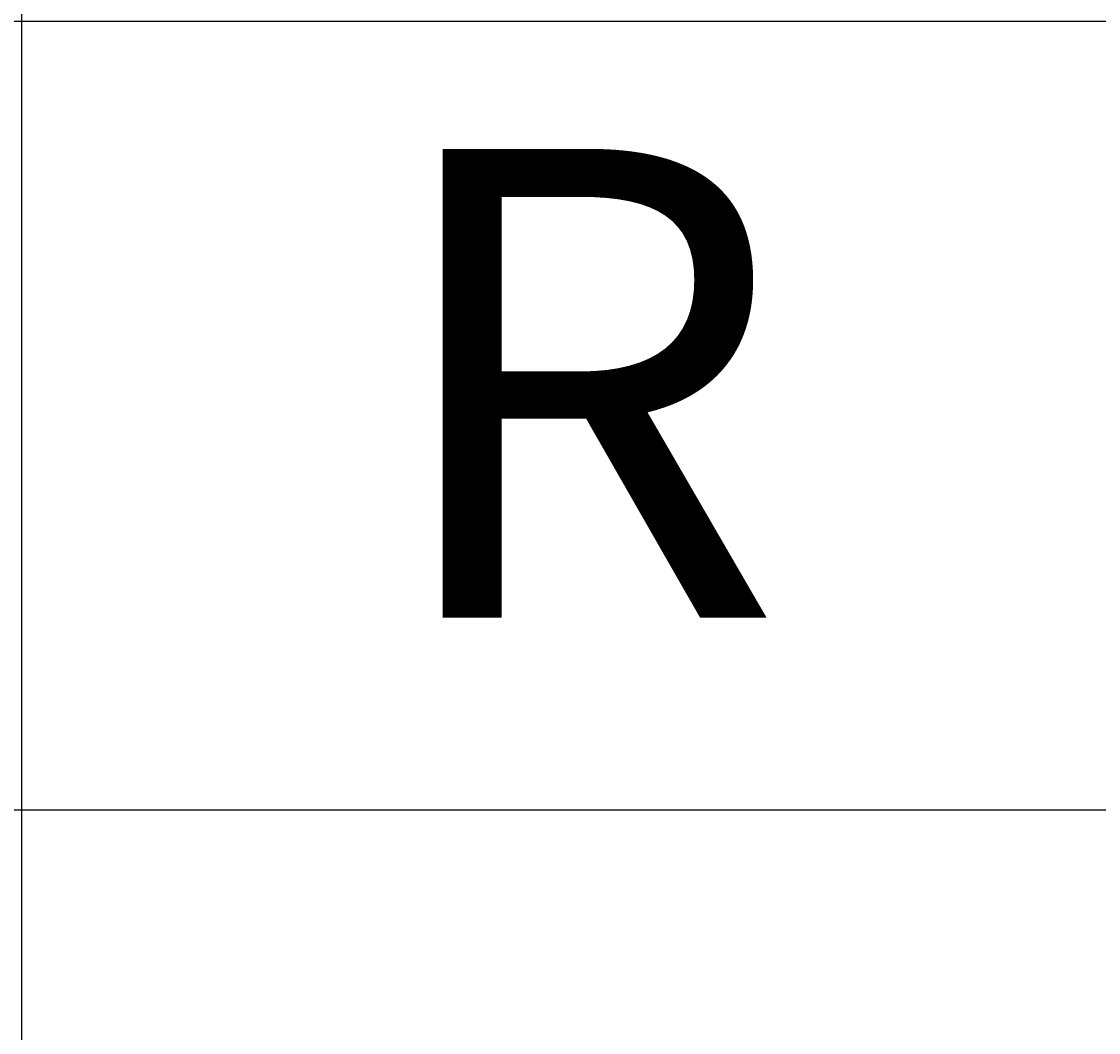
# Model space of a CAD drawing. Units: inches. Extents: x 35362 to 73946, y 43607 to 67532.
# Tile 134 of 134: x 67327 to 67834, y 59646 to 60122. Entities that reach past the tile are written whole.
import ezdxf

# ---------------------------------------------------------------- set-up
doc = ezdxf.new("R2010")
doc.units = ezdxf.units.IN
doc.header["$MEASUREMENT"] = 0
for name, color, linetype, lineweight in [('A-ANNO-DIMS', 2, 'Continuous', 18), ('E-ANNO-TEXT', 5, 'Continuous', 18), ('E-WIRE', 3, 'Continuous', 25)]:
    doc.layers.add(name, color=color, linetype=linetype, lineweight=lineweight)
doc.styles.get("Standard").update_dxf_attribs({"font": 'arial.ttf'})
doc.dimstyles.get("Standard").update_dxf_attribs({"dimtxt": 0.18, "dimasz": 0.18, "dimexe": 0.18, "dimexo": 0.0625, "dimgap": 0.09, "dimtad": 0, "dimtih": 1, "dimtoh": 1, "dimdec": 4, "dimzin": 0, "dimdsep": 46, "dimtxsty": 'Standard', "dimcen": 0.09, "dimadec": 0, "dimazin": 0, "dimtfac": 1, "dimtdec": 4, "dimtofl": 0, "dimtmove": 0, "dimatfit": 3, "dimfxl": 1, "dimtolj": 1, "dimtzin": 0, "dimarcsym": 0})

# ---------------------------------------------------------------- blocks, each defined once
blk = doc.blocks.new('*D8')
at = {"layer": 'A-ANNO-DIMS', "color": 0, "lineweight": -2, "transparency": 16777216}
for p, q in [((66271.28651900003, 65771.51172800003), (73945.82566600003, 65771.51172800003)), ((73945.64566600005, 65771.33172800003), (73945.64566600005, 59737.03093663782)), ((73945.64566600005, 53702.36633900002), (73945.64566600005, 59736.66713036224)), ((72185.70816600003, 53702.18633900003), (73945.82566600003, 53702.18633900003))]:
    blk.add_line(p, q, dxfattribs=at)
at = {"layer": 'A-ANNO-DIMS', "color": 0, "transparency": 16777216}
for points in [[(73945.61566600006, 65771.33172800003), (73945.67566600005, 65771.33172800003), (73945.64566600005, 65771.51172800003)], [(73945.61566600006, 53702.36633900002), (73945.67566600005, 53702.36633900002), (73945.64566600005, 53702.18633900003)]]:
    blk.add_solid(points, dxfattribs=at)
at = {"layer": 'Defpoints', "color": 0, "transparency": 16777216}
for p in [(66271.22401900003, 65771.51172800003), (73945.64566600005, 65771.51172800003), (72185.64566600003, 53702.18633900003)]:
    blk.add_point(p, dxfattribs=at)
at = {"layer": 'A-ANNO-DIMS', "color": 0, "transparency": 16777216, "insert": (73945.64566600005, 59736.84903349999), "char_height": 0.18, "attachment_point": 5}
blk.add_mtext('\\A1;12069', dxfattribs=at)
blk = doc.blocks.new('*D35')
at = {"layer": 'A-ANNO-DIMS', "color": 0, "lineweight": -2, "transparency": 16777216}
for p, q in [((61240.907336, 59185.206457), (61240.907336, 67531.691728)), ((61241.08733599999, 67531.51172799998), (64780.42646373397, 67531.51172799998)), ((68320.69076200001, 67531.51172799998), (64781.35163426603, 67531.51172799998)), ((68320.870762, 60122.408832), (68320.870762, 67531.691728))]:
    blk.add_line(p, q, dxfattribs=at)
at = {"layer": 'A-ANNO-DIMS', "color": 0, "transparency": 16777216}
for points in [[(61241.08733599999, 67531.541728), (61241.08733599999, 67531.481728), (61240.907336, 67531.51172799998)], [(68320.69076200001, 67531.541728), (68320.69076200001, 67531.481728), (68320.870762, 67531.51172799998)]]:
    blk.add_solid(points, dxfattribs=at)
at = {"layer": 'Defpoints', "color": 0, "transparency": 16777216}
for p in [(68320.870762, 67531.51172799998), (68320.870762, 60122.346332), (61240.907336, 59185.14395699999)]:
    blk.add_point(p, dxfattribs=at)
at = {"layer": 'A-ANNO-DIMS', "color": 0, "transparency": 16777216, "insert": (64780.889049, 67531.51172799998), "char_height": 0.18, "attachment_point": 5}
blk.add_mtext('\\A1;7080.0', dxfattribs=at)
blk = doc.blocks.new('*D36')
at = {"layer": 'A-ANNO-DIMS', "color": 0, "lineweight": -2, "transparency": 16777216}
for p, q in [((68320.80826200004, 60122.34633200002), (35361.76908500003, 60122.34633200002)), ((35361.94908500003, 60122.16633200002), (35361.94908500003, 57247.82893113781)), ((35361.94908500003, 54373.12772400002), (35361.94908500003, 57247.46512486223)), ((68320.80826200004, 54372.94772400003), (35361.76908500003, 54372.94772400002))]:
    blk.add_line(p, q, dxfattribs=at)
at = {"layer": 'A-ANNO-DIMS', "color": 0, "transparency": 16777216}
for points in [[(35361.91908500003, 60122.16633200002), (35361.97908500003, 60122.16633200002), (35361.94908500003, 60122.34633200002)], [(35361.91908500003, 54373.12772400002), (35361.97908500003, 54373.12772400002), (35361.94908500003, 54372.94772400002)]]:
    blk.add_solid(points, dxfattribs=at)
at = {"layer": 'Defpoints', "color": 0, "transparency": 16777216}
for p in [(68320.87076200004, 60122.34633200002), (35361.94908500003, 54372.94772400002), (68320.87076200004, 54372.94772400003)]:
    blk.add_point(p, dxfattribs=at)
at = {"layer": 'A-ANNO-DIMS', "color": 0, "transparency": 16777216, "insert": (35361.94908500004, 57247.64702799999), "char_height": 0.18, "attachment_point": 5}
blk.add_mtext('\\A1;5749.4', dxfattribs=at)
blk = doc.blocks.new('*D65')
at = {"layer": 'A-ANNO-DIMS', "color": 0, "lineweight": -2, "transparency": 16777216}
for p, q in [((65336.01600799999, 61293.223552), (65336.01600799999, 43606.678996)), ((67326.639741, 61293.223552), (67326.639741, 43606.678996)), ((65336.19600799999, 43606.858996), (66330.87277900206, 43606.858996)), ((67326.45974100001, 43606.858996), (66331.78296999796, 43606.858996))]:
    blk.add_line(p, q, dxfattribs=at)
at = {"layer": 'A-ANNO-DIMS', "color": 0, "transparency": 16777216}
for points in [[(65336.19600799999, 43606.888996), (65336.19600799999, 43606.828996), (65336.01600799999, 43606.858996)], [(67326.45974100001, 43606.888996), (67326.45974100001, 43606.828996), (67326.639741, 43606.858996)]]:
    blk.add_solid(points, dxfattribs=at)
at = {"layer": 'Defpoints', "color": 0, "transparency": 16777216}
for p in [(65336.01600799999, 61293.286052), (67326.639741, 61293.286052), (67326.639741, 43606.858996)]:
    blk.add_point(p, dxfattribs=at)
at = {"layer": 'A-ANNO-DIMS', "color": 0, "transparency": 16777216, "insert": (66331.32787450001, 43606.858996), "char_height": 0.18, "attachment_point": 5}
blk.add_mtext('\\A1;1990.6', dxfattribs=at)
blk = doc.blocks.new('*D70')
at = {"layer": 'A-ANNO-DIMS', "color": 0, "lineweight": -2, "transparency": 16777216}
for p, q in [((60785.27513900002, 64923.75242000003), (73945.82566600003, 64923.75242000003)), ((73945.64566600005, 64923.57242000003), (73945.64566600005, 62054.63015302935)), ((73945.64566600005, 59185.32395700003), (73945.64566600005, 62054.26622397069)), ((61240.96983600002, 59185.14395700003), (73945.82566600003, 59185.14395700003))]:
    blk.add_line(p, q, dxfattribs=at)
at = {"layer": 'A-ANNO-DIMS', "color": 0, "transparency": 16777216}
for points in [[(73945.61566600006, 64923.57242000003), (73945.67566600005, 64923.57242000003), (73945.64566600005, 64923.75242000003)], [(73945.61566600006, 59185.32395700003), (73945.67566600005, 59185.32395700003), (73945.64566600005, 59185.14395700003)]]:
    blk.add_solid(points, dxfattribs=at)
at = {"layer": 'Defpoints', "color": 0, "transparency": 16777216}
for p in [(60785.21263900002, 64923.75242000003), (73945.64566600005, 64923.75242000003), (61240.90733600002, 59185.14395700003)]:
    blk.add_point(p, dxfattribs=at)
at = {"layer": 'A-ANNO-DIMS', "color": 0, "transparency": 16777216, "insert": (73945.64566600005, 62054.44818849999), "char_height": 0.18, "attachment_point": 5}
blk.add_mtext('\\A1;5738.6', dxfattribs=at)
blk = doc.blocks.new('*D71')
at = {"layer": 'A-ANNO-DIMS', "color": 0, "lineweight": -2, "transparency": 16777216}
for p, q in [((63159.24181700003, 64828.55626700002), (73945.82566600003, 64828.55626700002)), ((73945.64566600005, 64828.37626700002), (73945.64566600005, 62007.03207652936)), ((73945.64566600005, 59185.32395700003), (73945.64566600005, 62006.6681474707)), ((61240.96983600002, 59185.14395700003), (73945.82566600003, 59185.14395700003))]:
    blk.add_line(p, q, dxfattribs=at)
at = {"layer": 'A-ANNO-DIMS', "color": 0, "transparency": 16777216}
for points in [[(73945.61566600006, 64828.37626700002), (73945.67566600005, 64828.37626700002), (73945.64566600005, 64828.55626700002)], [(73945.61566600006, 59185.32395700003), (73945.67566600005, 59185.32395700003), (73945.64566600005, 59185.14395700003)]]:
    blk.add_solid(points, dxfattribs=at)
at = {"layer": 'Defpoints', "color": 0, "transparency": 16777216}
for p in [(63159.17931700003, 64828.55626700002), (73945.64566600005, 64828.55626700002), (61240.90733600002, 59185.14395700003)]:
    blk.add_point(p, dxfattribs=at)
at = {"layer": 'A-ANNO-DIMS', "color": 0, "transparency": 16777216, "insert": (73945.64566600005, 62006.85011199999), "char_height": 0.18, "attachment_point": 5}
blk.add_mtext('\\A1;5643.4', dxfattribs=at)

msp = doc.modelspace()

# ---------------------------------------------------------------- linework, layer by layer
at = {"layer": 'E-WIRE'}
msp.add_line((68320.87076221016, 59750.68874003685), (64849.6346681835, 59750.68874003685), dxfattribs=at)

# ---------------------------------------------------------------- texts
at = {"layer": 'E-ANNO-TEXT'}
msp.add_text('R', height=220.8659825270206, dxfattribs=at).set_placement((67494.60997568478, 59841.47233897126))

# ---------------------------------------------------------------- dimensions: what is measured, and where the dimension line sits
at = {"layer": 'A-ANNO-DIMS'}
for base, p1, p2, picture, middle in [((68320.870762, 67531.51172799998), (61240.907336, 59185.14395699999), (68320.870762, 60122.346332), '*D35', (64780.889049, 67531.51172799998)), ((67326.639741, 43606.858996), (65336.01600799999, 61293.286052), (67326.639741, 61293.286052), '*D65', (66331.32787450001, 43606.858996))]:
    dim = msp.add_linear_dim(base=base, p1=p1, p2=p2, dimstyle='Standard', override={"dimdec": 1, "dimlfac": 1, "dimrnd": 0, "dimzin": 0, "dimdsep": 46, "dimlunit": 2}, dxfattribs=at)
    dim.commit()
    dim.dimension.update_dxf_attribs({"geometry": picture, "text_midpoint": middle})
for base, p1, p2, override, picture, middle in [((73945.64566600005, 65771.51172800003), (72185.645666, 53702.186339), (66271.224019, 65771.51172799998), {"dimdec": 0, "dimlfac": 1, "dimrnd": 0, "dimzin": 0, "dimdsep": 46, "dimlunit": 2}, '*D8', (73945.64566600005, 59736.84903349999)), ((73945.64566600005, 64923.75242000003), (61240.907336, 59185.14395699999), (60785.21263899999, 64923.75241999999), {"dimdec": 1, "dimlfac": 1, "dimrnd": 0, "dimzin": 0, "dimdsep": 46, "dimlunit": 2}, '*D70', (73945.64566600005, 62054.44818849999)), ((73945.64566600005, 64828.55626700002), (61240.907336, 59185.14395699999), (63159.179317, 64828.556267), {"dimdec": 1, "dimlfac": 1, "dimrnd": 0, "dimzin": 0, "dimdsep": 46, "dimlunit": 2}, '*D71', (73945.64566600005, 62006.85011199999)), ((35361.94908500003, 54372.94772400002), (68320.870762, 60122.346332), (68320.870762, 54372.947724), {"dimdec": 1, "dimlfac": 1, "dimrnd": 0, "dimzin": 0, "dimdsep": 46, "dimlunit": 2}, '*D36', (35361.94908500004, 57247.64702799999))]:
    dim = msp.add_linear_dim(base=base, p1=p1, p2=p2, angle=90, dimstyle='Standard', override=override, dxfattribs=at)
    dim.commit()
    dim.dimension.update_dxf_attribs({"geometry": picture, "text_midpoint": middle})

doc.saveas('drawing.dxf')
